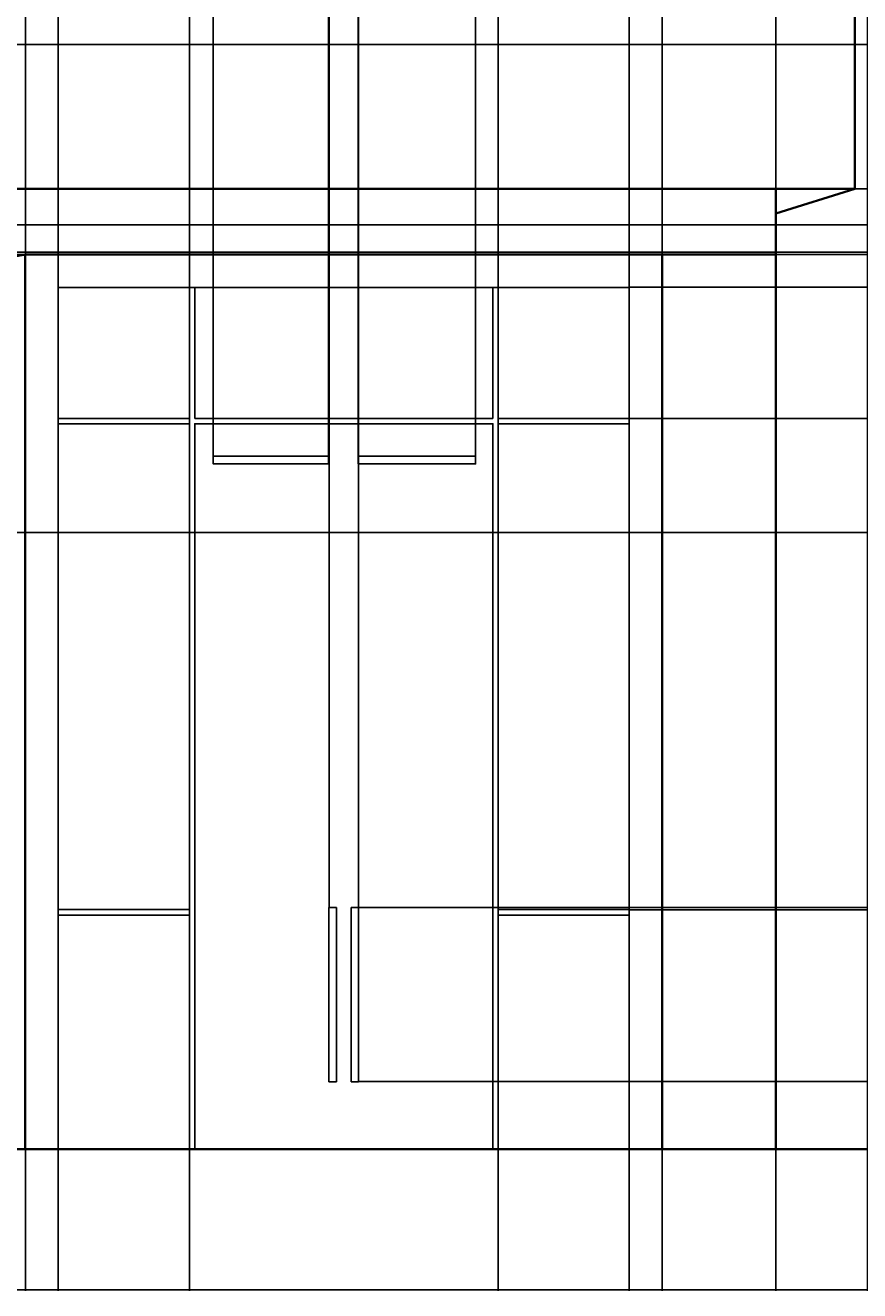
# Model space of a CAD drawing. Units: feet. Extents: x 4092 to 5585, y 725 to 1390.
# Tile 3 of 7: x 5022 to 5204, y 725 to 1001. Entities that reach past the tile are written whole.
import ezdxf

# ---------------------------------------------------------------- set-up
doc = ezdxf.new("R2010")
doc.units = ezdxf.units.FT
for name, color, linetype, lineweight in [('A-ANNO-DIMS', 2, 'Continuous', 18), ('A-DOOR', 3, 'Continuous', 25), ('A-ELEV', 7, 'Continuous', 35)]:
    doc.layers.add(name, color=color, linetype=linetype, lineweight=lineweight)
doc.styles.get("Standard").update_dxf_attribs({"font": 'arial.ttf'})
doc.dimstyles.get("Standard").update_dxf_attribs({"dimtxt": 0.18, "dimasz": 0.18, "dimexe": 0.18, "dimexo": 0.0625, "dimgap": 0.09, "dimtad": 0, "dimtih": 1, "dimtoh": 1, "dimdec": 1, "dimzin": 0, "dimdsep": 46, "dimlunit": 3, "dimtxsty": 'Standard', "dimcen": 0.09, "dimadec": 0, "dimazin": 0, "dimtfac": 1, "dimtdec": 1, "dimtofl": 0, "dimtmove": 0, "dimatfit": 3, "dimfxl": 1, "dimtolj": 1, "dimtzin": 0, "dimarcsym": 0})

# ---------------------------------------------------------------- blocks, each defined once
blk = doc.blocks.new('*D4')
at = {"layer": 'A-ANNO-DIMS', "color": 0, "lineweight": -2, "transparency": 16777216}
for p, q in [((4953.29, 755.89), (4953.29, 725.07)), ((5553.29, 755.89), (5553.29, 725.07)), ((4953.47, 725.25), (5253, 725.25)), ((5553.11, 725.25), (5253.58, 725.25))]:
    blk.add_line(p, q, dxfattribs=at)
at = {"layer": 'A-ANNO-DIMS', "color": 0, "transparency": 16777216}
for points in [[(4953.47, 725.28), (4953.47, 725.22), (4953.29, 725.25)], [(5553.11, 725.28), (5553.11, 725.22), (5553.29, 725.25)]]:
    blk.add_solid(points, dxfattribs=at)
at = {"layer": 'Defpoints', "color": 0, "transparency": 16777216}
for p in [(4953.29, 755.95), (5553.29, 755.95), (5553.29, 725.25)]:
    blk.add_point(p, dxfattribs=at)
at = {"layer": 'A-ANNO-DIMS', "color": 0, "transparency": 16777216, "insert": (5253.29, 725.25), "char_height": 0.18, "attachment_point": 5}
blk.add_mtext('\\A1;600', dxfattribs=at)
blk = doc.blocks.new('*D17')
at = {"layer": 'A-ANNO-DIMS', "color": 0, "lineweight": -2, "transparency": 16777216}
for p, q in [((5021.54, 951.2), (4921.27, 951.2)), ((4921.45, 951.02), (4921.45, 853.76)), ((4921.45, 756.13), (4921.45, 853.39)), ((5285.73, 755.95), (4921.27, 755.95))]:
    blk.add_line(p, q, dxfattribs=at)
at = {"layer": 'A-ANNO-DIMS', "color": 0, "transparency": 16777216}
for points in [[(4921.42, 951.02), (4921.48, 951.02), (4921.45, 951.2)], [(4921.42, 756.13), (4921.48, 756.13), (4921.45, 755.95)]]:
    blk.add_solid(points, dxfattribs=at)
at = {"layer": 'Defpoints', "color": 0, "transparency": 16777216}
for p in [(4921.45, 951.2), (5021.61, 951.2), (5285.79, 755.95)]:
    blk.add_point(p, dxfattribs=at)
at = {"layer": 'A-ANNO-DIMS', "color": 0, "transparency": 16777216, "insert": (4921.45, 853.58), "char_height": 0.18, "attachment_point": 5}
blk.add_mtext('\\A1;195.25', dxfattribs=at)
blk = doc.blocks.new('*D26')
at = {"layer": 'A-ANNO-DIMS', "color": 0, "lineweight": -2, "transparency": 16777216}
for p, q in [((5021.61, 755.89), (5021.61, 725.07)), ((5028.8, 755.89), (5028.8, 725.07)), ((5021.79, 725.25), (5024.81, 725.25)), ((5028.62, 725.25), (5025.6, 725.25))]:
    blk.add_line(p, q, dxfattribs=at)
at = {"layer": 'A-ANNO-DIMS', "color": 0, "transparency": 16777216}
for points in [[(5021.79, 725.28), (5021.79, 725.22), (5021.61, 725.25)], [(5028.62, 725.28), (5028.62, 725.22), (5028.8, 725.25)]]:
    blk.add_solid(points, dxfattribs=at)
at = {"layer": 'Defpoints', "color": 0, "transparency": 16777216}
for p in [(5021.61, 755.95), (5028.8, 755.95), (5028.8, 725.25)]:
    blk.add_point(p, dxfattribs=at)
at = {"layer": 'A-ANNO-DIMS', "color": 0, "transparency": 16777216, "insert": (5025.2, 725.25), "char_height": 0.18, "attachment_point": 5}
blk.add_mtext('\\A1;7.194', dxfattribs=at)
blk = doc.blocks.new('*D27')
at = {"layer": 'A-ANNO-DIMS', "color": 0, "lineweight": -2, "transparency": 16777216}
for p, q in [((5028.8, 755.89), (5028.8, 725.07)), ((5057.39, 755.89), (5057.39, 725.07)), ((5028.98, 725.25), (5042.7, 725.25)), ((5057.21, 725.25), (5043.49, 725.25))]:
    blk.add_line(p, q, dxfattribs=at)
at = {"layer": 'A-ANNO-DIMS', "color": 0, "transparency": 16777216}
for points in [[(5028.98, 725.28), (5028.98, 725.22), (5028.8, 725.25)], [(5057.21, 725.28), (5057.21, 725.22), (5057.39, 725.25)]]:
    blk.add_solid(points, dxfattribs=at)
at = {"layer": 'Defpoints', "color": 0, "transparency": 16777216}
for p in [(5028.8, 755.95), (5057.39, 755.95), (5057.39, 725.25)]:
    blk.add_point(p, dxfattribs=at)
at = {"layer": 'A-ANNO-DIMS', "color": 0, "transparency": 16777216, "insert": (5043.1, 725.25), "char_height": 0.18, "attachment_point": 5}
blk.add_mtext('\\A1;28.59', dxfattribs=at)
blk = doc.blocks.new('*D28')
at = {"layer": 'A-ANNO-DIMS', "color": 0, "lineweight": -2, "transparency": 16777216}
for p, q in [((5057.39, 755.89), (5057.39, 725.07)), ((5124.75, 755.89), (5124.75, 725.07)), ((5057.57, 725.25), (5090.68, 725.25)), ((5124.57, 725.25), (5091.46, 725.25))]:
    blk.add_line(p, q, dxfattribs=at)
at = {"layer": 'A-ANNO-DIMS', "color": 0, "transparency": 16777216}
for points in [[(5057.57, 725.28), (5057.57, 725.22), (5057.39, 725.25)], [(5124.57, 725.28), (5124.57, 725.22), (5124.75, 725.25)]]:
    blk.add_solid(points, dxfattribs=at)
at = {"layer": 'Defpoints', "color": 0, "transparency": 16777216}
for p in [(5057.39, 755.95), (5124.75, 755.95), (5124.75, 725.25)]:
    blk.add_point(p, dxfattribs=at)
at = {"layer": 'A-ANNO-DIMS', "color": 0, "transparency": 16777216, "insert": (5091.07, 725.25), "char_height": 0.18, "attachment_point": 5}
blk.add_mtext('\\A1;67.36', dxfattribs=at)
blk = doc.blocks.new('*D29')
at = {"layer": 'A-ANNO-DIMS', "color": 0, "lineweight": -2, "transparency": 16777216}
for p, q in [((5124.75, 755.89), (5124.75, 725.07)), ((5153.34, 755.89), (5153.34, 725.07)), ((5124.93, 725.25), (5138.65, 725.25)), ((5153.16, 725.25), (5139.44, 725.25))]:
    blk.add_line(p, q, dxfattribs=at)
at = {"layer": 'A-ANNO-DIMS', "color": 0, "transparency": 16777216}
for points in [[(5124.93, 725.28), (5124.93, 725.22), (5124.75, 725.25)], [(5153.16, 725.28), (5153.16, 725.22), (5153.34, 725.25)]]:
    blk.add_solid(points, dxfattribs=at)
at = {"layer": 'Defpoints', "color": 0, "transparency": 16777216}
for p in [(5124.75, 755.95), (5153.34, 755.95), (5153.34, 725.25)]:
    blk.add_point(p, dxfattribs=at)
at = {"layer": 'A-ANNO-DIMS', "color": 0, "transparency": 16777216, "insert": (5139.04, 725.25), "char_height": 0.18, "attachment_point": 5}
blk.add_mtext('\\A1;28.59', dxfattribs=at)
blk = doc.blocks.new('*D30')
at = {"layer": 'A-ANNO-DIMS', "color": 0, "lineweight": -2, "transparency": 16777216}
for p, q in [((5153.34, 755.89), (5153.34, 725.07)), ((5160.53, 755.89), (5160.53, 725.07)), ((5153.52, 725.25), (5156.54, 725.25)), ((5160.35, 725.25), (5157.33, 725.25))]:
    blk.add_line(p, q, dxfattribs=at)
at = {"layer": 'A-ANNO-DIMS', "color": 0, "transparency": 16777216}
for points in [[(5153.52, 725.28), (5153.52, 725.22), (5153.34, 725.25)], [(5160.35, 725.28), (5160.35, 725.22), (5160.53, 725.25)]]:
    blk.add_solid(points, dxfattribs=at)
at = {"layer": 'Defpoints', "color": 0, "transparency": 16777216}
for p in [(5153.34, 755.95), (5160.53, 755.95), (5160.53, 725.25)]:
    blk.add_point(p, dxfattribs=at)
at = {"layer": 'A-ANNO-DIMS', "color": 0, "transparency": 16777216, "insert": (5156.94, 725.25), "char_height": 0.18, "attachment_point": 5}
blk.add_mtext('\\A1;7.194', dxfattribs=at)
blk = doc.blocks.new('*D31')
at = {"layer": 'A-ANNO-DIMS', "color": 0, "lineweight": -2, "transparency": 16777216}
for p, q in [((5160.53, 755.89), (5160.53, 725.07)), ((5185.33, 755.89), (5185.33, 725.07)), ((5160.71, 725.25), (5172.47, 725.25)), ((5185.15, 725.25), (5173.4, 725.25))]:
    blk.add_line(p, q, dxfattribs=at)
at = {"layer": 'A-ANNO-DIMS', "color": 0, "transparency": 16777216}
for points in [[(5160.71, 725.28), (5160.71, 725.22), (5160.53, 725.25)], [(5185.15, 725.28), (5185.15, 725.22), (5185.33, 725.25)]]:
    blk.add_solid(points, dxfattribs=at)
at = {"layer": 'Defpoints', "color": 0, "transparency": 16777216}
for p in [(5160.53, 755.95), (5185.33, 755.95), (5185.33, 725.25)]:
    blk.add_point(p, dxfattribs=at)
at = {"layer": 'A-ANNO-DIMS', "color": 0, "transparency": 16777216, "insert": (5172.93, 725.25), "char_height": 0.18, "attachment_point": 5}
blk.add_mtext('\\A1;24.796', dxfattribs=at)
blk = doc.blocks.new('*D32')
at = {"layer": 'A-ANNO-DIMS', "color": 0, "lineweight": -2, "transparency": 16777216}
for p, q in [((5185.33, 755.89), (5185.33, 725.07)), ((5231.15, 755.89), (5231.15, 725.07)), ((5185.51, 725.25), (5207.84, 725.25)), ((5230.97, 725.25), (5208.64, 725.25))]:
    blk.add_line(p, q, dxfattribs=at)
at = {"layer": 'A-ANNO-DIMS', "color": 0, "transparency": 16777216}
for points in [[(5185.51, 725.28), (5185.51, 725.22), (5185.33, 725.25)], [(5230.97, 725.28), (5230.97, 725.22), (5231.15, 725.25)]]:
    blk.add_solid(points, dxfattribs=at)
at = {"layer": 'Defpoints', "color": 0, "transparency": 16777216}
for p in [(5185.33, 755.95), (5231.15, 755.95), (5231.15, 725.25)]:
    blk.add_point(p, dxfattribs=at)
at = {"layer": 'A-ANNO-DIMS', "color": 0, "transparency": 16777216, "insert": (5208.24, 725.25), "char_height": 0.18, "attachment_point": 5}
blk.add_mtext('\\A1;45.82', dxfattribs=at)
blk = doc.blocks.new('*D33')
at = {"layer": 'A-ANNO-DIMS', "color": 0, "lineweight": -2, "transparency": 16777216}
for p, q in [((5153.4, 808.21), (5584.71, 808.21)), ((5584.53, 808.03), (5584.53, 782.26)), ((5584.53, 756.13), (5584.53, 781.9)), ((5153.4, 755.95), (5584.71, 755.95))]:
    blk.add_line(p, q, dxfattribs=at)
at = {"layer": 'A-ANNO-DIMS', "color": 0, "transparency": 16777216}
for points in [[(5584.5, 808.03), (5584.56, 808.03), (5584.53, 808.21)], [(5584.5, 756.13), (5584.56, 756.13), (5584.53, 755.95)]]:
    blk.add_solid(points, dxfattribs=at)
at = {"layer": 'Defpoints', "color": 0, "transparency": 16777216}
for p in [(5153.34, 808.21), (5584.53, 808.21), (5153.34, 755.95)]:
    blk.add_point(p, dxfattribs=at)
at = {"layer": 'A-ANNO-DIMS', "color": 0, "transparency": 16777216, "insert": (5584.53, 782.08), "char_height": 0.18, "attachment_point": 5}
blk.add_mtext('\\A1;52.27', dxfattribs=at)
blk = doc.blocks.new('*D34')
at = {"layer": 'A-ANNO-DIMS', "color": 0, "lineweight": -2, "transparency": 16777216}
for p, q in [((5153.4, 915.42), (5584.71, 915.42)), ((5584.53, 915.24), (5584.53, 862)), ((5584.53, 808.39), (5584.53, 861.63)), ((5153.4, 808.21), (5584.71, 808.21))]:
    blk.add_line(p, q, dxfattribs=at)
at = {"layer": 'A-ANNO-DIMS', "color": 0, "transparency": 16777216}
for points in [[(5584.5, 915.24), (5584.56, 915.24), (5584.53, 915.42)], [(5584.5, 808.39), (5584.56, 808.39), (5584.53, 808.21)]]:
    blk.add_solid(points, dxfattribs=at)
at = {"layer": 'Defpoints', "color": 0, "transparency": 16777216}
for p in [(5153.34, 915.42), (5584.53, 915.42), (5153.34, 808.21)]:
    blk.add_point(p, dxfattribs=at)
at = {"layer": 'A-ANNO-DIMS', "color": 0, "transparency": 16777216, "insert": (5584.53, 861.82), "char_height": 0.18, "attachment_point": 5}
blk.add_mtext('\\A1;107.2', dxfattribs=at)
blk = doc.blocks.new('*D35')
at = {"layer": 'A-ANNO-DIMS', "color": 0, "lineweight": -2, "transparency": 16777216}
for p, q in [((5153.4, 944.01), (5584.71, 944.01)), ((5584.53, 943.83), (5584.53, 929.9)), ((5584.53, 915.6), (5584.53, 929.53)), ((5153.4, 915.42), (5584.71, 915.42))]:
    blk.add_line(p, q, dxfattribs=at)
at = {"layer": 'A-ANNO-DIMS', "color": 0, "transparency": 16777216}
for points in [[(5584.5, 943.83), (5584.56, 943.83), (5584.53, 944.01)], [(5584.5, 915.6), (5584.56, 915.6), (5584.53, 915.42)]]:
    blk.add_solid(points, dxfattribs=at)
at = {"layer": 'Defpoints', "color": 0, "transparency": 16777216}
for p in [(5153.34, 944.01), (5584.53, 944.01), (5153.34, 915.42)]:
    blk.add_point(p, dxfattribs=at)
at = {"layer": 'A-ANNO-DIMS', "color": 0, "transparency": 16777216, "insert": (5584.53, 929.71), "char_height": 0.18, "attachment_point": 5}
blk.add_mtext('\\A1;28.59', dxfattribs=at)
blk = doc.blocks.new('*D36')
at = {"layer": 'A-ANNO-DIMS', "color": 0, "lineweight": -2, "transparency": 16777216}
for p, q in [((5160.6, 951.2), (5584.71, 951.2)), ((5584.53, 951.02), (5584.53, 947.79)), ((5584.53, 944.19), (5584.53, 947.42)), ((5153.4, 944.01), (5584.71, 944.01))]:
    blk.add_line(p, q, dxfattribs=at)
at = {"layer": 'A-ANNO-DIMS', "color": 0, "transparency": 16777216}
for points in [[(5584.5, 951.02), (5584.56, 951.02), (5584.53, 951.2)], [(5584.5, 944.19), (5584.56, 944.19), (5584.53, 944.01)]]:
    blk.add_solid(points, dxfattribs=at)
at = {"layer": 'Defpoints', "color": 0, "transparency": 16777216}
for p in [(5160.53, 951.2), (5584.53, 951.2), (5153.34, 944.01)]:
    blk.add_point(p, dxfattribs=at)
at = {"layer": 'A-ANNO-DIMS', "color": 0, "transparency": 16777216, "insert": (5584.53, 947.61), "char_height": 0.18, "attachment_point": 5}
blk.add_mtext('\\A1;7.194', dxfattribs=at)
blk = doc.blocks.new('*D37')
at = {"layer": 'A-ANNO-DIMS', "color": 0, "lineweight": -2, "transparency": 16777216}
for p, q in [((5094.36, 770.68), (5584.71, 770.68)), ((5584.53, 770.5), (5584.53, 763.5)), ((5584.53, 756.13), (5584.53, 763.13)), ((5057.45, 755.95), (5584.71, 755.95))]:
    blk.add_line(p, q, dxfattribs=at)
at = {"layer": 'A-ANNO-DIMS', "color": 0, "transparency": 16777216}
for points in [[(5584.5, 770.5), (5584.56, 770.5), (5584.53, 770.68)], [(5584.5, 756.13), (5584.56, 756.13), (5584.53, 755.95)]]:
    blk.add_solid(points, dxfattribs=at)
at = {"layer": 'Defpoints', "color": 0, "transparency": 16777216}
for p in [(5094.3, 770.68), (5584.53, 770.68), (5057.39, 755.95)]:
    blk.add_point(p, dxfattribs=at)
at = {"layer": 'A-ANNO-DIMS', "color": 0, "transparency": 16777216, "insert": (5584.53, 763.31), "char_height": 0.18, "attachment_point": 5}
blk.add_mtext('\\A1;14.73', dxfattribs=at)
blk = doc.blocks.new('*D38')
at = {"layer": 'A-ANNO-DIMS', "color": 0, "lineweight": -2, "transparency": 16777216}
for p, q in [((5094.36, 808.65), (5584.71, 808.65)), ((5584.53, 808.47), (5584.53, 789.85)), ((5584.53, 770.86), (5584.53, 789.48)), ((5094.36, 770.68), (5584.71, 770.68))]:
    blk.add_line(p, q, dxfattribs=at)
at = {"layer": 'A-ANNO-DIMS', "color": 0, "transparency": 16777216}
for points in [[(5584.5, 808.47), (5584.56, 808.47), (5584.53, 808.65)], [(5584.5, 770.86), (5584.56, 770.86), (5584.53, 770.68)]]:
    blk.add_solid(points, dxfattribs=at)
at = {"layer": 'Defpoints', "color": 0, "transparency": 16777216}
for p in [(5094.3, 808.65), (5584.53, 808.65), (5094.3, 770.68)]:
    blk.add_point(p, dxfattribs=at)
at = {"layer": 'A-ANNO-DIMS', "color": 0, "transparency": 16777216, "insert": (5584.53, 789.67), "char_height": 0.18, "attachment_point": 5}
blk.add_mtext('\\A1;37.97', dxfattribs=at)
blk = doc.blocks.new('*D39')
at = {"layer": 'A-ANNO-DIMS', "color": 0, "lineweight": -2, "transparency": 16777216}
for p, q in [((5087.84, 808.72), (5087.84, 1389.85)), ((5088.02, 1389.67), (5090.69, 1389.67)), ((5094.12, 1389.67), (5091.45, 1389.67)), ((5094.3, 808.72), (5094.3, 1389.85))]:
    blk.add_line(p, q, dxfattribs=at)
at = {"layer": 'A-ANNO-DIMS', "color": 0, "transparency": 16777216}
for points in [[(5088.02, 1389.7), (5088.02, 1389.64), (5087.84, 1389.67)], [(5094.12, 1389.7), (5094.12, 1389.64), (5094.3, 1389.67)]]:
    blk.add_solid(points, dxfattribs=at)
at = {"layer": 'Defpoints', "color": 0, "transparency": 16777216}
for p in [(5094.3, 1389.67), (5087.84, 808.65), (5094.3, 808.65)]:
    blk.add_point(p, dxfattribs=at)
at = {"layer": 'A-ANNO-DIMS', "color": 0, "transparency": 16777216, "insert": (5091.07, 1389.67), "char_height": 0.18, "attachment_point": 5}
blk.add_mtext('\\A1;6.461', dxfattribs=at)
blk = doc.blocks.new('*D40')
at = {"layer": 'A-ANNO-DIMS', "color": 0, "lineweight": -2, "transparency": 16777216}
for p, q in [((5062.58, 907.22), (5062.58, 1389.85)), ((5062.76, 1389.67), (5074.7, 1389.67)), ((5087.57, 1389.67), (5075.63, 1389.67)), ((5087.75, 907.22), (5087.75, 1389.85))]:
    blk.add_line(p, q, dxfattribs=at)
at = {"layer": 'A-ANNO-DIMS', "color": 0, "transparency": 16777216}
for points in [[(5062.76, 1389.7), (5062.76, 1389.64), (5062.58, 1389.67)], [(5087.57, 1389.7), (5087.57, 1389.64), (5087.75, 1389.67)]]:
    blk.add_solid(points, dxfattribs=at)
at = {"layer": 'Defpoints', "color": 0, "transparency": 16777216}
for p in [(5087.75, 1389.67), (5062.58, 907.16), (5087.75, 907.16)]:
    blk.add_point(p, dxfattribs=at)
at = {"layer": 'A-ANNO-DIMS', "color": 0, "transparency": 16777216, "insert": (5075.16, 1389.67), "char_height": 0.18, "attachment_point": 5}
blk.add_mtext('\\A1;25.164', dxfattribs=at)
blk = doc.blocks.new('*D41')
at = {"layer": 'A-ANNO-DIMS', "color": 0, "lineweight": -2, "transparency": 16777216}
for p, q in [((5087.75, 907.22), (5087.75, 1389.85)), ((5087.93, 1389.67), (5090.59, 1389.67)), ((5094.04, 1389.67), (5091.38, 1389.67)), ((5094.22, 907.22), (5094.22, 1389.85))]:
    blk.add_line(p, q, dxfattribs=at)
at = {"layer": 'A-ANNO-DIMS', "color": 0, "transparency": 16777216}
for points in [[(5087.93, 1389.7), (5087.93, 1389.64), (5087.75, 1389.67)], [(5094.04, 1389.7), (5094.04, 1389.64), (5094.22, 1389.67)]]:
    blk.add_solid(points, dxfattribs=at)
at = {"layer": 'Defpoints', "color": 0, "transparency": 16777216}
for p in [(5094.22, 1389.67), (5087.75, 907.16), (5094.22, 907.16)]:
    blk.add_point(p, dxfattribs=at)
at = {"layer": 'A-ANNO-DIMS', "color": 0, "transparency": 16777216, "insert": (5090.98, 1389.67), "char_height": 0.18, "attachment_point": 5}
blk.add_mtext('\\A1;6.474', dxfattribs=at)
blk = doc.blocks.new('*D42')
at = {"layer": 'A-ANNO-DIMS', "color": 0, "lineweight": -2, "transparency": 16777216}
for p, q in [((5094.22, 907.22), (5094.22, 1389.85)), ((5094.4, 1389.67), (5106.69, 1389.67)), ((5119.64, 1389.67), (5107.34, 1389.67)), ((5119.82, 907.22), (5119.82, 1389.85))]:
    blk.add_line(p, q, dxfattribs=at)
at = {"layer": 'A-ANNO-DIMS', "color": 0, "transparency": 16777216}
for points in [[(5094.4, 1389.7), (5094.4, 1389.64), (5094.22, 1389.67)], [(5119.64, 1389.7), (5119.64, 1389.64), (5119.82, 1389.67)]]:
    blk.add_solid(points, dxfattribs=at)
at = {"layer": 'Defpoints', "color": 0, "transparency": 16777216}
for p in [(5119.82, 1389.67), (5094.22, 907.16), (5119.82, 907.16)]:
    blk.add_point(p, dxfattribs=at)
at = {"layer": 'A-ANNO-DIMS', "color": 0, "transparency": 16777216, "insert": (5107.02, 1389.67), "char_height": 0.18, "attachment_point": 5}
blk.add_mtext('\\A1;25.6', dxfattribs=at)
blk = doc.blocks.new('*D50')
at = {"layer": 'A-ANNO-DIMS', "color": 0, "lineweight": -2, "transparency": 16777216}
for p, q in [((5021.61, 1010.73), (5021.61, 725.07)), ((5028.8, 1010.73), (5028.8, 725.07)), ((5021.79, 725.25), (5024.81, 725.25)), ((5028.62, 725.25), (5025.6, 725.25))]:
    blk.add_line(p, q, dxfattribs=at)
at = {"layer": 'A-ANNO-DIMS', "color": 0, "transparency": 16777216}
for points in [[(5021.79, 725.28), (5021.79, 725.22), (5021.61, 725.25)], [(5028.62, 725.28), (5028.62, 725.22), (5028.8, 725.25)]]:
    blk.add_solid(points, dxfattribs=at)
at = {"layer": 'Defpoints', "color": 0, "transparency": 16777216}
for p in [(5021.61, 1010.79), (5028.8, 1010.79), (5028.8, 725.25)]:
    blk.add_point(p, dxfattribs=at)
at = {"layer": 'A-ANNO-DIMS', "color": 0, "transparency": 16777216, "insert": (5025.2, 725.25), "char_height": 0.18, "attachment_point": 5}
blk.add_mtext('\\A1;7.194', dxfattribs=at)
blk = doc.blocks.new('*D51')
at = {"layer": 'A-ANNO-DIMS', "color": 0, "lineweight": -2, "transparency": 16777216}
for p, q in [((5028.8, 1010.73), (5028.8, 725.07)), ((5057.39, 1010.73), (5057.39, 725.07)), ((5028.98, 725.25), (5042.7, 725.25)), ((5057.21, 725.25), (5043.49, 725.25))]:
    blk.add_line(p, q, dxfattribs=at)
at = {"layer": 'A-ANNO-DIMS', "color": 0, "transparency": 16777216}
for points in [[(5028.98, 725.28), (5028.98, 725.22), (5028.8, 725.25)], [(5057.21, 725.28), (5057.21, 725.22), (5057.39, 725.25)]]:
    blk.add_solid(points, dxfattribs=at)
at = {"layer": 'Defpoints', "color": 0, "transparency": 16777216}
for p in [(5028.8, 1010.79), (5057.39, 1010.79), (5057.39, 725.25)]:
    blk.add_point(p, dxfattribs=at)
at = {"layer": 'A-ANNO-DIMS', "color": 0, "transparency": 16777216, "insert": (5043.1, 725.25), "char_height": 0.18, "attachment_point": 5}
blk.add_mtext('\\A1;28.59', dxfattribs=at)
blk = doc.blocks.new('*D52')
at = {"layer": 'A-ANNO-DIMS', "color": 0, "lineweight": -2, "transparency": 16777216}
for p, q in [((5057.39, 1010.73), (5057.39, 725.07)), ((5124.75, 1010.73), (5124.75, 725.07)), ((5057.57, 725.25), (5090.68, 725.25)), ((5124.57, 725.25), (5091.46, 725.25))]:
    blk.add_line(p, q, dxfattribs=at)
at = {"layer": 'A-ANNO-DIMS', "color": 0, "transparency": 16777216}
for points in [[(5057.57, 725.28), (5057.57, 725.22), (5057.39, 725.25)], [(5124.57, 725.28), (5124.57, 725.22), (5124.75, 725.25)]]:
    blk.add_solid(points, dxfattribs=at)
at = {"layer": 'Defpoints', "color": 0, "transparency": 16777216}
for p in [(5057.39, 1010.79), (5124.75, 1010.79), (5124.75, 725.25)]:
    blk.add_point(p, dxfattribs=at)
at = {"layer": 'A-ANNO-DIMS', "color": 0, "transparency": 16777216, "insert": (5091.07, 725.25), "char_height": 0.18, "attachment_point": 5}
blk.add_mtext('\\A1;67.36', dxfattribs=at)
blk = doc.blocks.new('*D53')
at = {"layer": 'A-ANNO-DIMS', "color": 0, "lineweight": -2, "transparency": 16777216}
for p, q in [((5124.75, 1010.73), (5124.75, 725.07)), ((5153.34, 1010.73), (5153.34, 725.07)), ((5124.93, 725.25), (5138.65, 725.25)), ((5153.16, 725.25), (5139.44, 725.25))]:
    blk.add_line(p, q, dxfattribs=at)
at = {"layer": 'A-ANNO-DIMS', "color": 0, "transparency": 16777216}
for points in [[(5124.93, 725.28), (5124.93, 725.22), (5124.75, 725.25)], [(5153.16, 725.28), (5153.16, 725.22), (5153.34, 725.25)]]:
    blk.add_solid(points, dxfattribs=at)
at = {"layer": 'Defpoints', "color": 0, "transparency": 16777216}
for p in [(5124.75, 1010.79), (5153.34, 1010.79), (5153.34, 725.25)]:
    blk.add_point(p, dxfattribs=at)
at = {"layer": 'A-ANNO-DIMS', "color": 0, "transparency": 16777216, "insert": (5139.04, 725.25), "char_height": 0.18, "attachment_point": 5}
blk.add_mtext('\\A1;28.59', dxfattribs=at)
blk = doc.blocks.new('*D54')
at = {"layer": 'A-ANNO-DIMS', "color": 0, "lineweight": -2, "transparency": 16777216}
for p, q in [((5153.34, 1010.73), (5153.34, 725.07)), ((5160.53, 1010.73), (5160.53, 725.07)), ((5153.52, 725.25), (5156.54, 725.25)), ((5160.35, 725.25), (5157.33, 725.25))]:
    blk.add_line(p, q, dxfattribs=at)
at = {"layer": 'A-ANNO-DIMS', "color": 0, "transparency": 16777216}
for points in [[(5153.52, 725.28), (5153.52, 725.22), (5153.34, 725.25)], [(5160.35, 725.28), (5160.35, 725.22), (5160.53, 725.25)]]:
    blk.add_solid(points, dxfattribs=at)
at = {"layer": 'Defpoints', "color": 0, "transparency": 16777216}
for p in [(5153.34, 1010.79), (5160.53, 1010.79), (5160.53, 725.25)]:
    blk.add_point(p, dxfattribs=at)
at = {"layer": 'A-ANNO-DIMS', "color": 0, "transparency": 16777216, "insert": (5156.94, 725.25), "char_height": 0.18, "attachment_point": 5}
blk.add_mtext('\\A1;7.194', dxfattribs=at)
blk = doc.blocks.new('*D55')
at = {"layer": 'A-ANNO-DIMS', "color": 0, "lineweight": -2, "transparency": 16777216}
for p, q in [((5160.53, 1010.73), (5160.53, 725.07)), ((5185.33, 1010.73), (5185.33, 725.07)), ((5160.71, 725.25), (5172.47, 725.25)), ((5185.15, 725.25), (5173.4, 725.25))]:
    blk.add_line(p, q, dxfattribs=at)
at = {"layer": 'A-ANNO-DIMS', "color": 0, "transparency": 16777216}
for points in [[(5160.71, 725.28), (5160.71, 725.22), (5160.53, 725.25)], [(5185.15, 725.28), (5185.15, 725.22), (5185.33, 725.25)]]:
    blk.add_solid(points, dxfattribs=at)
at = {"layer": 'Defpoints', "color": 0, "transparency": 16777216}
for p in [(5160.53, 1010.79), (5185.33, 1010.79), (5185.33, 725.25)]:
    blk.add_point(p, dxfattribs=at)
at = {"layer": 'A-ANNO-DIMS', "color": 0, "transparency": 16777216, "insert": (5172.93, 725.25), "char_height": 0.18, "attachment_point": 5}
blk.add_mtext('\\A1;24.796', dxfattribs=at)
blk = doc.blocks.new('*D56')
at = {"layer": 'A-ANNO-DIMS', "color": 0, "lineweight": -2, "transparency": 16777216}
for p, q in [((5185.33, 1010.73), (5185.33, 725.07)), ((5205.28, 1010.73), (5205.28, 725.07)), ((5185.51, 725.25), (5194.85, 725.25)), ((5205.1, 725.25), (5195.76, 725.25))]:
    blk.add_line(p, q, dxfattribs=at)
at = {"layer": 'A-ANNO-DIMS', "color": 0, "transparency": 16777216}
for points in [[(5185.51, 725.28), (5185.51, 725.22), (5185.33, 725.25)], [(5205.1, 725.28), (5205.1, 725.22), (5205.28, 725.25)]]:
    blk.add_solid(points, dxfattribs=at)
at = {"layer": 'Defpoints', "color": 0, "transparency": 16777216}
for p in [(5185.33, 1010.79), (5205.28, 1010.79), (5205.28, 725.25)]:
    blk.add_point(p, dxfattribs=at)
at = {"layer": 'A-ANNO-DIMS', "color": 0, "transparency": 16777216, "insert": (5195.3, 725.25), "char_height": 0.18, "attachment_point": 5}
blk.add_mtext('\\A1;19.947', dxfattribs=at)
blk = doc.blocks.new('*D71')
at = {"layer": 'A-ANNO-DIMS', "color": 0, "lineweight": -2, "transparency": 16777216}
for p, q in [((5285.73, 890.54), (4921.27, 890.54)), ((4921.45, 890.36), (4921.45, 823.43)), ((4921.45, 756.13), (4921.45, 823.06)), ((5285.73, 755.95), (4921.27, 755.95))]:
    blk.add_line(p, q, dxfattribs=at)
at = {"layer": 'A-ANNO-DIMS', "color": 0, "transparency": 16777216}
for points in [[(4921.42, 890.36), (4921.48, 890.36), (4921.45, 890.54)], [(4921.42, 756.13), (4921.48, 756.13), (4921.45, 755.95)]]:
    blk.add_solid(points, dxfattribs=at)
at = {"layer": 'Defpoints', "color": 0, "transparency": 16777216}
for p in [(4921.45, 890.54), (5285.79, 890.54), (5285.79, 755.95)]:
    blk.add_point(p, dxfattribs=at)
at = {"layer": 'A-ANNO-DIMS', "color": 0, "transparency": 16777216, "insert": (4921.45, 823.24), "char_height": 0.18, "attachment_point": 5}
blk.add_mtext('\\A1;134.6', dxfattribs=at)
blk = doc.blocks.new('*D72')
at = {"layer": 'A-ANNO-DIMS', "color": 0, "lineweight": -2, "transparency": 16777216}
for p, q in [((5285.73, 996.97), (4921.27, 996.97)), ((4921.45, 996.79), (4921.45, 943.94)), ((4921.45, 890.72), (4921.45, 943.57)), ((5285.73, 890.54), (4921.27, 890.54))]:
    blk.add_line(p, q, dxfattribs=at)
at = {"layer": 'A-ANNO-DIMS', "color": 0, "transparency": 16777216}
for points in [[(4921.42, 996.79), (4921.48, 996.79), (4921.45, 996.97)], [(4921.42, 890.72), (4921.48, 890.72), (4921.45, 890.54)]]:
    blk.add_solid(points, dxfattribs=at)
at = {"layer": 'Defpoints', "color": 0, "transparency": 16777216}
for p in [(4921.45, 996.97), (5285.79, 996.97), (5285.79, 890.54)]:
    blk.add_point(p, dxfattribs=at)
at = {"layer": 'A-ANNO-DIMS', "color": 0, "transparency": 16777216, "insert": (4921.45, 943.75), "char_height": 0.18, "attachment_point": 5}
blk.add_mtext('\\A1;106.43', dxfattribs=at)
blk = doc.blocks.new('*D75')
at = {"layer": 'A-ANNO-DIMS', "color": 0, "lineweight": -2, "transparency": 16777216}
for p, q in [((5392.49, 951.65), (4921.27, 951.65)), ((4921.45, 951.47), (4921.45, 853.98)), ((4921.45, 756.13), (4921.45, 853.62)), ((5392.49, 755.95), (4921.27, 755.95))]:
    blk.add_line(p, q, dxfattribs=at)
at = {"layer": 'A-ANNO-DIMS', "color": 0, "transparency": 16777216}
for points in [[(4921.42, 951.47), (4921.48, 951.47), (4921.45, 951.65)], [(4921.42, 756.13), (4921.48, 756.13), (4921.45, 755.95)]]:
    blk.add_solid(points, dxfattribs=at)
at = {"layer": 'Defpoints', "color": 0, "transparency": 16777216}
for p in [(4921.45, 951.65), (5392.55, 951.65), (5392.55, 755.95)]:
    blk.add_point(p, dxfattribs=at)
at = {"layer": 'A-ANNO-DIMS', "color": 0, "transparency": 16777216, "insert": (4921.45, 853.8), "char_height": 0.18, "attachment_point": 5}
blk.add_mtext('\\A1;195.7', dxfattribs=at)
blk = doc.blocks.new('*D76')
at = {"layer": 'A-ANNO-DIMS', "color": 0, "lineweight": -2, "transparency": 16777216}
for p, q in [((5392.49, 957.65), (4921.27, 957.65)), ((4921.45, 957.47), (4921.45, 954.83)), ((4921.45, 951.83), (4921.45, 954.46)), ((5392.49, 951.65), (4921.27, 951.65))]:
    blk.add_line(p, q, dxfattribs=at)
at = {"layer": 'A-ANNO-DIMS', "color": 0, "transparency": 16777216}
for points in [[(4921.42, 957.47), (4921.48, 957.47), (4921.45, 957.65)], [(4921.42, 951.83), (4921.48, 951.83), (4921.45, 951.65)]]:
    blk.add_solid(points, dxfattribs=at)
at = {"layer": 'Defpoints', "color": 0, "transparency": 16777216}
for p in [(4921.45, 957.65), (5392.55, 957.65), (5392.55, 951.65)]:
    blk.add_point(p, dxfattribs=at)
at = {"layer": 'A-ANNO-DIMS', "color": 0, "transparency": 16777216, "insert": (4921.45, 954.65), "char_height": 0.18, "attachment_point": 5}
blk.add_mtext('\\A1;6', dxfattribs=at)
blk = doc.blocks.new('*D77')
at = {"layer": 'A-ANNO-DIMS', "color": 0, "lineweight": -2, "transparency": 16777216}
for p, q in [((5392.49, 965.48), (4921.27, 965.48)), ((4921.45, 965.3), (4921.45, 961.74)), ((4921.45, 957.83), (4921.45, 961.38)), ((5392.49, 957.65), (4921.27, 957.65))]:
    blk.add_line(p, q, dxfattribs=at)
at = {"layer": 'A-ANNO-DIMS', "color": 0, "transparency": 16777216}
for points in [[(4921.42, 965.3), (4921.48, 965.3), (4921.45, 965.48)], [(4921.42, 957.83), (4921.48, 957.83), (4921.45, 957.65)]]:
    blk.add_solid(points, dxfattribs=at)
at = {"layer": 'Defpoints', "color": 0, "transparency": 16777216}
for p in [(4921.45, 965.48), (5392.55, 965.48), (5392.55, 957.65)]:
    blk.add_point(p, dxfattribs=at)
at = {"layer": 'A-ANNO-DIMS', "color": 0, "transparency": 16777216, "insert": (4921.45, 961.56), "char_height": 0.18, "attachment_point": 5}
blk.add_mtext('\\A1;7.833', dxfattribs=at)
blk = doc.blocks.new('*D78')
at = {"layer": 'A-ANNO-DIMS', "color": 0, "lineweight": -2, "transparency": 16777216}
for p, q in [((5392.49, 1007.95), (4921.27, 1007.95)), ((4921.45, 1007.77), (4921.45, 986.89)), ((4921.45, 965.66), (4921.45, 986.53)), ((5392.49, 965.48), (4921.27, 965.48))]:
    blk.add_line(p, q, dxfattribs=at)
at = {"layer": 'A-ANNO-DIMS', "color": 0, "transparency": 16777216}
for points in [[(4921.42, 1007.77), (4921.48, 1007.77), (4921.45, 1007.95)], [(4921.42, 965.66), (4921.48, 965.66), (4921.45, 965.48)]]:
    blk.add_solid(points, dxfattribs=at)
at = {"layer": 'Defpoints', "color": 0, "transparency": 16777216}
for p in [(4921.45, 1007.95), (5392.55, 1007.95), (5392.55, 965.48)]:
    blk.add_point(p, dxfattribs=at)
at = {"layer": 'A-ANNO-DIMS', "color": 0, "transparency": 16777216, "insert": (4921.45, 986.71), "char_height": 0.18, "attachment_point": 5}
blk.add_mtext('\\A1;42.47', dxfattribs=at)

msp = doc.modelspace()

# ---------------------------------------------------------------- linework, layer by layer
at = {"layer": 'A-DOOR'}
for p, q in [((5057.3906, 915.418), (5057.3906, 944.0084)), ((5058.5615, 915.418), (5058.5615, 944.0084)), ((5123.5775, 915.418), (5123.5775, 944.0084)), ((5124.7484, 915.418), (5124.7484, 944.0084)), ((5057.3906, 915.418), (5028.8002, 915.418)), ((5057.3906, 914.2471), (5028.8002, 914.2471)), ((5124.7484, 915.418), (5153.3388, 915.418)), ((5124.7484, 914.2471), (5153.3388, 914.2471)), ((5057.3906, 808.2143), (5028.8002, 808.2143)), ((5057.3906, 807.0434), (5028.8002, 807.0434)), ((5124.7484, 808.2143), (5153.3388, 808.2143)), ((5124.7484, 807.0434), (5153.3388, 807.0434))]:
    msp.add_line(p, q, dxfattribs=at)
for points in [[(5028.8002, 755.9488), (5028.8002, 944.0084), (5153.3388, 944.0084), (5153.3388, 755.9488)], [(5057.3906, 808.2143), (5057.3906, 914.2471)], [(5058.5615, 915.418), (5123.5775, 915.418)], [(5058.5615, 755.9488), (5058.5615, 914.2471), (5123.5775, 914.2471), (5123.5775, 755.9488)], [(5124.7484, 914.2471), (5124.7484, 808.2143)], [(5087.7457, 905.4904), (5062.5819, 905.4904), (5062.5819, 907.159), (5087.7457, 907.159)], [(5087.7457, 905.4904), (5087.7457, 907.159)], [(5094.2195, 907.159), (5119.8191, 907.159), (5119.8191, 905.4904), (5094.2195, 905.4904)], [(5094.2195, 907.159), (5094.2195, 905.4904)], [(5057.3906, 755.9488), (5057.3906, 807.0434)], [(5124.7484, 807.0434), (5124.7484, 755.9488)]]:
    msp.add_lwpolyline(points, dxfattribs=at)
for points in [[(5087.8389, 808.6527), (5089.4542, 808.6527), (5089.4542, 770.6797), (5087.8389, 770.6797)], [(5094.3002, 808.6527), (5092.6849, 808.6527), (5092.6849, 770.6797), (5094.3002, 770.6797)]]:
    msp.add_lwpolyline(points, close=True, dxfattribs=at)
at = {"layer": 'A-ELEV'}
for p, q in [((5202.5428, 965.4789), (5185.3285, 960.128)), ((4999.1145, 946.8601), (5021.6062, 951.2024)), ((5021.6062, 951.2024), (5185.3285, 951.2024)), ((4953.293, 755.9488), (5553.293, 755.9488))]:
    msp.add_line(p, q, dxfattribs=at)
for points in [[(4953.293, 755.9488), (5231.15, 755.9488), (5231.15, 1253.9488), (4953.293, 1253.9488)], [(4981.4448, 1007.9488), (5202.5428, 1007.9488), (5202.5428, 965.4789), (4981.4448, 965.4789)], [(5021.6062, 951.2024), (5160.5329, 951.2024), (5160.5329, 755.9488), (5021.6062, 755.9488)]]:
    msp.add_lwpolyline(points, close=True, dxfattribs=at)
msp.add_lwpolyline([(5185.3285, 755.9488), (5185.3285, 965.4789)], dxfattribs=at)

# ---------------------------------------------------------------- dimensions: what is measured, and where the dimension line sits
at = {"layer": 'A-ANNO-DIMS'}
for base, p1, p2, override, picture, middle in [((5087.7457, 1389.6731), (5062.5819, 907.159), (5087.7457, 907.159), {"dimdec": 3, "dimlfac": 1, "dimrnd": 0, "dimzin": 0, "dimdsep": 46, "dimlunit": 2}, '*D40', (5075.1638, 1389.6731)), ((5094.2195, 1389.6731), (5087.7457, 907.159), (5094.2195, 907.159), {"dimdec": 3, "dimlfac": 1, "dimrnd": 0, "dimzin": 0, "dimdsep": 46, "dimlunit": 2}, '*D41', (5090.9826, 1389.6731)), ((5094.3002, 1389.6731), (5087.8389, 808.6527), (5094.3002, 808.6527), {"dimdec": 3, "dimlfac": 1, "dimrnd": 0, "dimzin": 0, "dimdsep": 46, "dimlunit": 2}, '*D39', (5091.0695, 1389.6731)), ((5119.8191, 1389.6731), (5094.2195, 907.159), (5119.8191, 907.159), {"dimdec": 1, "dimlfac": 1, "dimrnd": 0, "dimzin": 0, "dimdsep": 46, "dimlunit": 2}, '*D42', (5107.0193, 1389.6731)), ((5028.8002, 725.2488), (5021.6062, 1010.7906), (5028.8002, 1010.7906), {"dimdec": 3, "dimlfac": 1, "dimrnd": 0, "dimzin": 0, "dimdsep": 46, "dimlunit": 2}, '*D50', (5025.2032, 725.2488)), ((5057.3906, 725.2488), (5028.8002, 1010.7906), (5057.3906, 1010.7906), {"dimdec": 2, "dimlfac": 1, "dimrnd": 0, "dimzin": 0, "dimdsep": 46, "dimlunit": 2}, '*D51', (5043.0954, 725.2488)), ((5124.7484, 725.2488), (5057.3906, 1010.7906), (5124.7484, 1010.7906), {"dimdec": 2, "dimlfac": 1, "dimrnd": 0, "dimzin": 0, "dimdsep": 46, "dimlunit": 2}, '*D52', (5091.0695, 725.2488)), ((5153.3388, 725.2488), (5124.7484, 1010.7906), (5153.3388, 1010.7906), {"dimdec": 2, "dimlfac": 1, "dimrnd": 0, "dimzin": 0, "dimdsep": 46, "dimlunit": 2}, '*D53', (5139.0436, 725.2488)), ((5160.5329, 725.2488), (5153.3388, 1010.7906), (5160.5329, 1010.7906), {"dimdec": 3, "dimlfac": 1, "dimrnd": 0, "dimzin": 0, "dimdsep": 46, "dimlunit": 2}, '*D54', (5156.9359, 725.2488)), ((5185.3285, 725.2488), (5160.5329, 1010.7906), (5185.3285, 1010.7906), {"dimdec": 3, "dimlfac": 1, "dimrnd": 0, "dimzin": 0, "dimdsep": 46, "dimlunit": 2}, '*D55', (5172.9307, 725.2488)), ((5205.2757, 725.2488), (5185.3285, 1010.7906), (5205.2757, 1010.7906), {"dimdec": 3, "dimlfac": 1, "dimrnd": 0, "dimzin": 0, "dimdsep": 46, "dimlunit": 2}, '*D56', (5195.3021, 725.2488)), ((5553.293, 725.2488), (4953.293, 755.9488), (5553.293, 755.9488), {"dimdec": 0, "dimlfac": 1, "dimrnd": 0, "dimzin": 0, "dimdsep": 46, "dimlunit": 2}, '*D4', (5253.293, 725.2488)), ((5028.8002, 725.2488), (5021.6062, 755.9488), (5028.8002, 755.9488), {"dimdec": 3, "dimlfac": 1, "dimrnd": 0, "dimzin": 0, "dimdsep": 46, "dimlunit": 2}, '*D26', (5025.2032, 725.2488)), ((5057.3906, 725.2488), (5028.8002, 755.9488), (5057.3906, 755.9488), {"dimdec": 2, "dimlfac": 1, "dimrnd": 0, "dimzin": 0, "dimdsep": 46, "dimlunit": 2}, '*D27', (5043.0954, 725.2488)), ((5124.7484, 725.2488), (5057.3906, 755.9488), (5124.7484, 755.9488), {"dimdec": 2, "dimlfac": 1, "dimrnd": 0, "dimzin": 0, "dimdsep": 46, "dimlunit": 2}, '*D28', (5091.0695, 725.2488)), ((5153.3388, 725.2488), (5124.7484, 755.9488), (5153.3388, 755.9488), {"dimdec": 2, "dimlfac": 1, "dimrnd": 0, "dimzin": 0, "dimdsep": 46, "dimlunit": 2}, '*D29', (5139.0436, 725.2488)), ((5160.5329, 725.2488), (5153.3388, 755.9488), (5160.5329, 755.9488), {"dimdec": 3, "dimlfac": 1, "dimrnd": 0, "dimzin": 0, "dimdsep": 46, "dimlunit": 2}, '*D30', (5156.9359, 725.2488)), ((5185.3285, 725.2488), (5160.5329, 755.9488), (5185.3285, 755.9488), {"dimdec": 3, "dimlfac": 1, "dimrnd": 0, "dimzin": 0, "dimdsep": 46, "dimlunit": 2}, '*D31', (5172.9307, 725.2488)), ((5231.15, 725.2488), (5185.3285, 755.9488), (5231.15, 755.9488), {"dimdec": 2, "dimlfac": 1, "dimrnd": 0, "dimzin": 0, "dimdsep": 46, "dimlunit": 2}, '*D32', (5208.2393, 725.2488))]:
    dim = msp.add_linear_dim(base=base, p1=p1, p2=p2, dimstyle='Standard', override=override, dxfattribs=at)
    dim.commit()
    dim.dimension.update_dxf_attribs({"geometry": picture, "text_midpoint": middle})
for base, p1, p2, override, picture, middle in [((4921.4517, 1007.9488), (5392.5521, 965.4789), (5392.5521, 1007.9488), {"dimdec": 2, "dimlfac": 1, "dimrnd": 0, "dimzin": 0, "dimdsep": 46, "dimlunit": 2}, '*D78', (4921.4517, 986.7139)), ((4921.4517, 996.9712), (5285.7915, 890.5384), (5285.7915, 996.9712), {"dimdec": 2, "dimlfac": 1, "dimrnd": 0, "dimzin": 0, "dimdsep": 46, "dimlunit": 2}, '*D72', (4921.4517, 943.7548)), ((4921.4517, 965.4789), (5392.5521, 957.6463), (5392.5521, 965.4789), {"dimdec": 3, "dimlfac": 1, "dimrnd": 0, "dimzin": 0, "dimdsep": 46, "dimlunit": 2}, '*D77', (4921.4517, 961.5626)), ((4921.4517, 957.6463), (5392.5521, 951.6463), (5392.5521, 957.6463), {"dimdec": 0, "dimlfac": 1, "dimrnd": 0, "dimzin": 0, "dimdsep": 46, "dimlunit": 2}, '*D76', (4921.4517, 954.6463)), ((4921.4517, 951.2024), (5285.7915, 755.9488), (5021.6062, 951.2024), {"dimdec": 2, "dimlfac": 1, "dimrnd": 0, "dimzin": 0, "dimdsep": 46, "dimlunit": 2}, '*D17', (4921.4517, 853.5756)), ((4921.4517, 951.6463), (5392.5521, 755.9488), (5392.5521, 951.6463), {"dimdec": 1, "dimlfac": 1, "dimrnd": 0, "dimzin": 0, "dimdsep": 46, "dimlunit": 2}, '*D75', (4921.4517, 853.7975)), ((5584.5322, 951.2024), (5153.3388, 944.0084), (5160.5329, 951.2024), {"dimdec": 3, "dimlfac": 1, "dimrnd": 0, "dimzin": 0, "dimdsep": 46, "dimlunit": 2}, '*D36', (5584.5322, 947.6054)), ((5584.5322, 944.0084), (5153.3388, 915.418), (5153.3388, 944.0084), {"dimdec": 2, "dimlfac": 1, "dimrnd": 0, "dimzin": 0, "dimdsep": 46, "dimlunit": 2}, '*D35', (5584.5322, 929.7132)), ((5584.5322, 915.418), (5153.3388, 808.2143), (5153.3388, 915.418), {"dimdec": 1, "dimlfac": 1, "dimrnd": 0, "dimzin": 0, "dimdsep": 46, "dimlunit": 2}, '*D34', (5584.5322, 861.8161)), ((4921.4517, 890.5384), (5285.7915, 755.9488), (5285.7915, 890.5384), {"dimdec": 1, "dimlfac": 1, "dimrnd": 0, "dimzin": 0, "dimdsep": 46, "dimlunit": 2}, '*D71', (4921.4517, 823.2436)), ((5584.5322, 808.6527), (5094.3002, 770.6797), (5094.3002, 808.6527), {"dimdec": 2, "dimlfac": 1, "dimrnd": 0, "dimzin": 0, "dimdsep": 46, "dimlunit": 2}, '*D38', (5584.5322, 789.6662)), ((5584.5322, 808.2143), (5153.3388, 755.9488), (5153.3388, 808.2143), {"dimdec": 2, "dimlfac": 1, "dimrnd": 0, "dimzin": 0, "dimdsep": 46, "dimlunit": 2}, '*D33', (5584.5322, 782.0815)), ((5584.5322, 770.6797), (5057.3906, 755.9488), (5094.3002, 770.6797), {"dimdec": 2, "dimlfac": 1, "dimrnd": 0, "dimzin": 0, "dimdsep": 46, "dimlunit": 2}, '*D37', (5584.5322, 763.3143))]:
    dim = msp.add_linear_dim(base=base, p1=p1, p2=p2, angle=90, dimstyle='Standard', override=override, dxfattribs=at)
    dim.commit()
    dim.dimension.update_dxf_attribs({"geometry": picture, "text_midpoint": middle})

doc.saveas('drawing.dxf')
